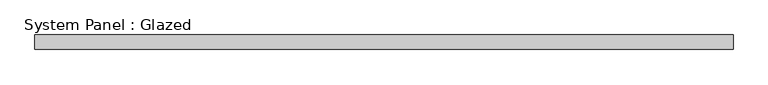
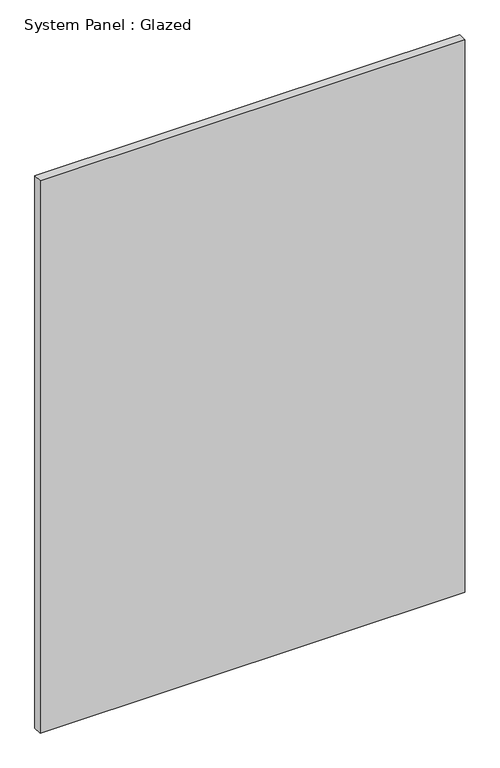
"""IFC4 building model written with IfcOpenShell, lengths in millimetres: plate geometry, System Panel : Glazed."""

from ifc_helpers import new_model, si_unit, origin, origin_with_axes, place, context, project, spatial, polyline, outline, extrude, source, transform, mapped, element, save


def system_panel_glazed_888d7767(model_context):
    return source(origin(), model_context, "Body", "SweptSolid", [
        extrude(outline(polyline([(609.5999999, 19.05), (-609.5999999, 19.05), (-609.5999999, 44.45), (609.5999999, 44.45), (609.5999999, 19.05)])), origin_with_axes(), (0.0, 0.0, 1.0), 1676.4),
    ])


if __name__ == "__main__":
    model = new_model("IFC4")
    model_context = context("Model", 3, world=origin())
    ifc_project = project(units=[si_unit("LENGTHUNIT", "METRE", prefix="MILLI")], contexts=[model_context])
    site = spatial("IfcSite", under=ifc_project)
    building = spatial("IfcBuilding", under=site)
    placement = place(None, origin())
    system_panel_glazed_shape = system_panel_glazed_888d7767(model_context)
    element("IfcPlate", 1, ObjectType="System Panel : Glazed", at=placement, inside=building, context=model_context, shape_type="MappedRepresentation", body=[
        mapped(system_panel_glazed_shape, transform((0.0, 0.0, 0.0), x_axis=(1.0, 0.0, 0.0), y_axis=(0.0, 1.0, 0.0), z_axis=(0.0, 0.0, 1.0))),
    ])
    save(model, "model.ifc")

# Revit data of these elements
# Type "System Panel : Glazed"
#   Construction Type Id = "GSP4R"
#   Analytic Construction = "1/8 in Pilkington single glazing"
#   Visual Light Transmittance = 0.9
#   Solar Heat Gain Coefficient = 0.86
#   Heat Transfer Coefficient (U) = 1.18115 BTU/(h·ft²·°F)
#   Define Thermal Properties by = 1
# Element 1 (IfcPlate, "System Panel : Glazed")
#   Materials on its faces: "Glass"
# Materials
#   "Glass": class "Glass", colour RGB 0 128 192, transparency 0.75, Description = "Soda Lime Glass", Cost = 0
